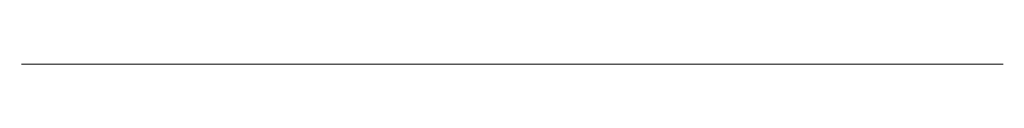
# Model space of a CAD drawing. Units: millimetres. Extents: x 393 to 526, y 0 to 0.
import ezdxf

# ---------------------------------------------------------------- set-up
doc = ezdxf.new("R2010")
doc.units = ezdxf.units.MM
doc.layers.add('M-CONS', color=8, linetype='Continuous', lineweight=13)

msp = doc.modelspace()

# ---------------------------------------------------------------- linework, layer by layer
at = {"layer": 'M-CONS', "extrusion": (0, -1, 0)}
for p, q in [((409.89, 0, 172.24), (414.4, 0, 176.74)), ((409.89, 0, 172.24), (413.42, 0, 168.7)), ((438.65, 0, 200.94), (440.73, 0, 195.31)), ((481.11, 0, 200.94), (479.03, 0, 195.31)), ((509.86, 0, 172.26), (506.32, 0, 168.72))]:
    msp.add_line(p, q, dxfattribs=at)
msp.add_lwpolyline([(516.97, 165.2), (525.4, 173.73, 1), (521.85, 177.25), (516.94, 172.28, -0.415518), (509.86, 172.26), (505.36, 176.74), (491.92, 190.15), (481.11, 200.94, 0.414214), (474.04, 200.93, -0.414902), (445.72, 200.93, 0.414214), (438.65, 200.94), (427.84, 190.15), (414.4, 176.74), (409.89, 172.24, -0.414214), (402.82, 172.25), (397.87, 177.21, 1), (394.33, 173.68), (394.33, 173.68), (402.81, 165.18), (402.81, 165.18, 0.414214), (409.88, 165.17), (409.88, 165.17), (438.94, 194.16, -0.365977), (445.37, 194.7, 0.319845), (474.39, 194.7, -0.365977), (480.82, 194.16), (509.88, 165.17), (509.88, 165.17, 0.414214), (516.95, 165.18), (516.95, 165.18)], format="xyb", dxfattribs=at)
for points in [[(414.4, 176.74), (408.13, 182.18, -1.05996), (422.07, 196.48), (427.84, 190.15)], [(505.36, 176.74), (511.63, 182.18, 1.05996), (497.69, 196.48), (491.92, 190.15)]]:
    msp.add_lwpolyline(points, format="xyb", close=True, dxfattribs=at)
for points in [[(431.21, 186.46), (431.32, 186.34)], [(488.54, 186.46), (488.44, 186.34)]]:
    msp.add_lwpolyline(points, dxfattribs=at)
for centre in [(414.68, 189.74), (505.08, 189.74)]:
    msp.add_circle(centre, 2.5, dxfattribs=at)

doc.saveas('drawing.dxf')
